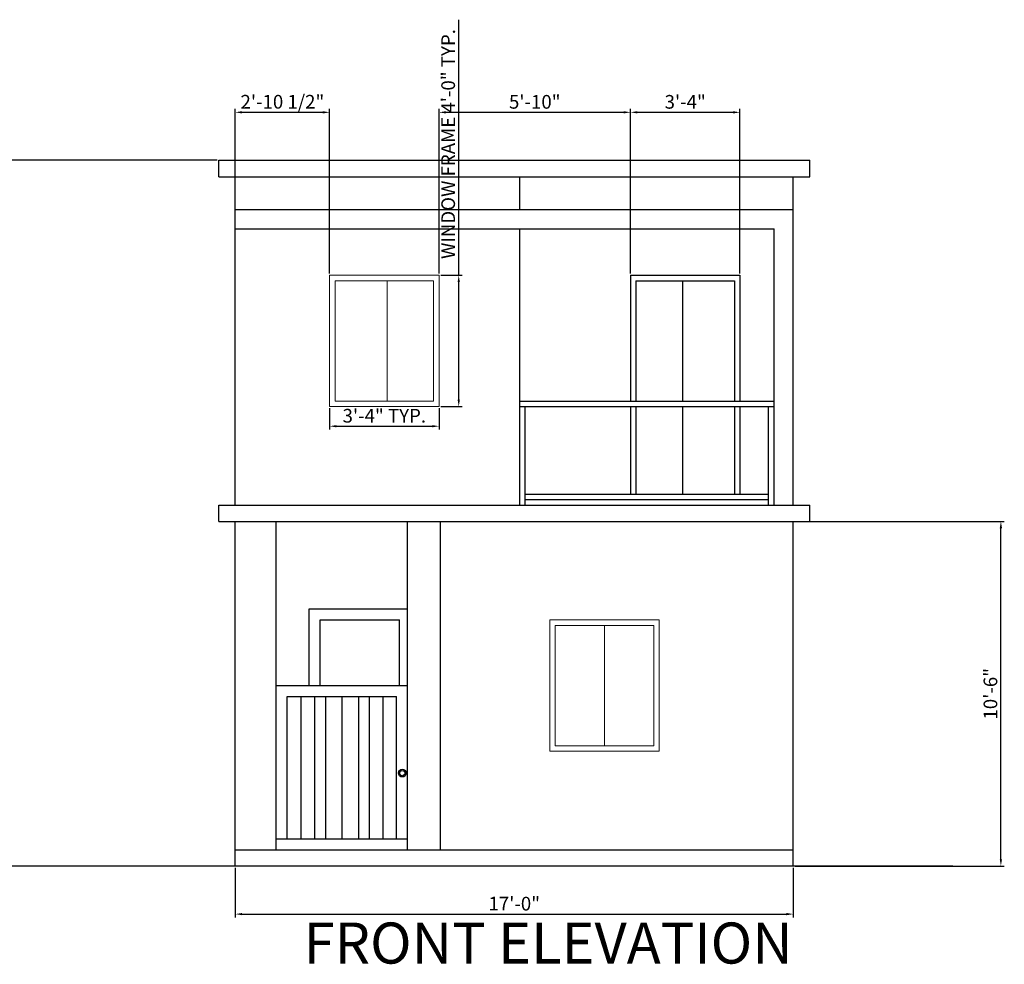
# Model space of a CAD drawing. Units: inches. Extents: x 1662 to 23131, y 1265 to 19127.
# Tile 17 of 26: x 20050 to 20410, y 8426 to 8771. Entities that reach past the tile are written whole.
import ezdxf

# ---------------------------------------------------------------- set-up
doc = ezdxf.new("R2010")
doc.units = ezdxf.units.IN
for name, color, linetype, lineweight in [('A-ANNO-DIMS', 4, 'Continuous', 18), ('A-ANNO-TITL', 7, 'Continuous', 35), ('A-ELEV', 7, 'Continuous', 25), ('A-ELEV-GLAZ', 4, 'Continuous', 18)]:
    doc.layers.add(name, color=color, linetype=linetype, lineweight=lineweight)
doc.styles.get("Standard").update_dxf_attribs({"font": 'arial.ttf'})
doc.dimstyles.new('ISO-25', dxfattribs={"dimtxt": 5, "dimasz": 2.5, "dimexe": 1.25, "dimexo": 0.625, "dimtad": 1, "dimlunit": 3, "dimtxsty": 'Standard', "dimcen": 2.5, "dimadec": 0, "dimazin": 0, "dimtfac": 1, "dimtmove": 0, "dimatfit": 3, "dimfxl": 1, "dimarcsym": 0})

# ---------------------------------------------------------------- blocks, each defined once
blk = doc.blocks.new('GLAZ-FRAME-ELEV-40X48')
for p, q in [((0, 48), (0, 0)), ((40, 48), (0, 48)), ((40, 48), (40, 0)), ((2, 46), (2, 2)), ((38, 46), (2, 46)), ((38, 46), (38, 2)), ((38, 2), (2, 2)), ((40, 0), (0, 0))]:
    blk.add_line(p, q)
blk = doc.blocks.new('*D195')
at = {"layer": 'A-ANNO-DIMS', "color": 0, "lineweight": -2, "transparency": 16777216}
for p, q in [((20210.7, 8677.94), (20210.7, 8771.35)), ((20204.13, 8677.94), (20211.95, 8677.94)), ((20210.7, 8632.44), (20210.7, 8675.44)), ((20204.13, 8629.94), (20211.95, 8629.94))]:
    blk.add_line(p, q, dxfattribs=at)
at = {"layer": 'A-ANNO-DIMS', "color": 0, "transparency": 16777216}
for points in [[(20210.29, 8675.44), (20211.12, 8675.44), (20210.7, 8677.94)], [(20210.29, 8632.44), (20211.12, 8632.44), (20210.7, 8629.94)]]:
    blk.add_solid(points, dxfattribs=at)
at = {"layer": 'Defpoints', "color": 0, "transparency": 16777216}
for p in [(20203.5, 8677.94), (20210.7, 8677.94), (20203.5, 8629.94)]:
    blk.add_point(p, dxfattribs=at)
at = {"layer": 'A-ANNO-DIMS', "color": 0, "transparency": 16777216, "insert": (20207.49, 8725.89), "char_height": 5, "attachment_point": 5, "rotation": 90}
blk.add_mtext('WINDOW FRAME 4\'-0" TYP.', dxfattribs=at)
blk = doc.blocks.new('*D196')
at = {"layer": 'A-ANNO-DIMS', "color": 0, "lineweight": -2, "transparency": 16777216}
for p, q in [((20163.5, 8629.31), (20163.5, 8621.49)), ((20203.5, 8629.31), (20203.5, 8621.49)), ((20166, 8622.74), (20201, 8622.74))]:
    blk.add_line(p, q, dxfattribs=at)
at = {"layer": 'A-ANNO-DIMS', "color": 0, "transparency": 16777216}
for points in [[(20166, 8623.16), (20166, 8622.32), (20163.5, 8622.74)], [(20201, 8623.16), (20201, 8622.32), (20203.5, 8622.74)]]:
    blk.add_solid(points, dxfattribs=at)
at = {"layer": 'Defpoints', "color": 0, "transparency": 16777216}
for p in [(20163.5, 8629.94), (20203.5, 8629.94), (20203.5, 8622.74)]:
    blk.add_point(p, dxfattribs=at)
at = {"layer": 'A-ANNO-DIMS', "color": 0, "transparency": 16777216, "insert": (20183.5, 8625.92), "char_height": 5, "attachment_point": 5}
blk.add_mtext('3\'-4" TYP.', dxfattribs=at)
blk = doc.blocks.new('*D245')
at = {"layer": 'A-ANNO-DIMS', "color": 0, "lineweight": -2, "transparency": 16777216}
for p, q in [((20129, 8461.31), (20129, 8443.14)), ((20333, 8461.31), (20333, 8443.14)), ((20131.5, 8444.39), (20330.5, 8444.39))]:
    blk.add_line(p, q, dxfattribs=at)
at = {"layer": 'A-ANNO-DIMS', "color": 0, "transparency": 16777216}
for points in [[(20131.5, 8444.81), (20131.5, 8443.97), (20129, 8444.39)], [(20330.5, 8444.81), (20330.5, 8443.97), (20333, 8444.39)]]:
    blk.add_solid(points, dxfattribs=at)
at = {"layer": 'Defpoints', "color": 0, "transparency": 16777216}
for p in [(20129, 8461.94), (20333, 8461.94), (20333, 8444.39)]:
    blk.add_point(p, dxfattribs=at)
at = {"layer": 'A-ANNO-DIMS', "color": 0, "transparency": 16777216, "insert": (20231, 8447.57), "char_height": 5, "attachment_point": 5}
blk.add_mtext('17\'-0"', dxfattribs=at)
blk = doc.blocks.new('*D246')
at = {"layer": 'A-ANNO-DIMS', "color": 0, "lineweight": -2, "transparency": 16777216}
for p, q in [((20122.38, 8719.94), (20031.81, 8719.94)), ((20033.06, 8464.44), (20033.06, 8717.44)), ((20128.38, 8461.94), (20031.81, 8461.94))]:
    blk.add_line(p, q, dxfattribs=at)
at = {"layer": 'A-ANNO-DIMS', "color": 0, "transparency": 16777216}
for points in [[(20032.64, 8717.44), (20033.48, 8717.44), (20033.06, 8719.94)], [(20032.64, 8464.44), (20033.48, 8464.44), (20033.06, 8461.94)]]:
    blk.add_solid(points, dxfattribs=at)
at = {"layer": 'Defpoints', "color": 0, "transparency": 16777216}
for p in [(20033.06, 8719.94), (20123, 8719.94), (20129, 8461.94)]:
    blk.add_point(p, dxfattribs=at)
at = {"layer": 'A-ANNO-DIMS', "color": 0, "transparency": 16777216, "insert": (20029.88, 8590.94), "char_height": 5, "attachment_point": 5, "rotation": 90}
blk.add_mtext('21\'-6"', dxfattribs=at)
blk = doc.blocks.new('*D247')
at = {"layer": 'A-ANNO-DIMS', "color": 0, "lineweight": -2, "transparency": 16777216}
for p, q in [((20333.63, 8587.94), (20410.14, 8587.94)), ((20408.89, 8464.44), (20408.89, 8585.44)), ((20333.63, 8461.94), (20410.14, 8461.94))]:
    blk.add_line(p, q, dxfattribs=at)
at = {"layer": 'A-ANNO-DIMS', "color": 0, "transparency": 16777216}
for points in [[(20408.48, 8585.44), (20409.31, 8585.44), (20408.89, 8587.94)], [(20408.48, 8464.44), (20409.31, 8464.44), (20408.89, 8461.94)]]:
    blk.add_solid(points, dxfattribs=at)
at = {"layer": 'Defpoints', "color": 0, "transparency": 16777216}
for p in [(20333, 8587.94), (20408.89, 8587.94), (20333, 8461.94)]:
    blk.add_point(p, dxfattribs=at)
at = {"layer": 'A-ANNO-DIMS', "color": 0, "transparency": 16777216, "insert": (20405.72, 8524.94), "char_height": 5, "attachment_point": 5, "rotation": 90}
blk.add_mtext('10\'-6"', dxfattribs=at)
blk = doc.blocks.new('*D248')
at = {"layer": 'A-ANNO-DIMS', "color": 0, "lineweight": -2, "transparency": 16777216}
for p, q in [((20203.5, 8678.56), (20203.5, 8738.74)), ((20206, 8737.49), (20271, 8737.49)), ((20273.5, 8678.56), (20273.5, 8738.74))]:
    blk.add_line(p, q, dxfattribs=at)
at = {"layer": 'A-ANNO-DIMS', "color": 0, "transparency": 16777216}
for points in [[(20206, 8737.91), (20206, 8737.07), (20203.5, 8737.49)], [(20271, 8737.91), (20271, 8737.07), (20273.5, 8737.49)]]:
    blk.add_solid(points, dxfattribs=at)
at = {"layer": 'Defpoints', "color": 0, "transparency": 16777216}
for p in [(20273.5, 8737.49), (20203.5, 8677.94), (20273.5, 8677.94)]:
    blk.add_point(p, dxfattribs=at)
at = {"layer": 'A-ANNO-DIMS', "color": 0, "transparency": 16777216, "insert": (20238.5, 8740.67), "char_height": 5, "attachment_point": 5}
blk.add_mtext('5\'-10"', dxfattribs=at)
blk = doc.blocks.new('*D249')
at = {"layer": 'A-ANNO-DIMS', "color": 0, "lineweight": -2, "transparency": 16777216}
for p, q in [((20129, 8695.56), (20129, 8738.74)), ((20131.5, 8737.49), (20161, 8737.49)), ((20163.5, 8678.56), (20163.5, 8738.74))]:
    blk.add_line(p, q, dxfattribs=at)
at = {"layer": 'A-ANNO-DIMS', "color": 0, "transparency": 16777216}
for points in [[(20131.5, 8737.91), (20131.5, 8737.07), (20129, 8737.49)], [(20161, 8737.91), (20161, 8737.07), (20163.5, 8737.49)]]:
    blk.add_solid(points, dxfattribs=at)
at = {"layer": 'Defpoints', "color": 0, "transparency": 16777216}
for p in [(20163.5, 8737.49), (20129, 8694.94), (20163.5, 8677.94)]:
    blk.add_point(p, dxfattribs=at)
at = {"layer": 'A-ANNO-DIMS', "color": 0, "transparency": 16777216, "insert": (20146.25, 8740.7), "char_height": 5, "attachment_point": 5}
blk.add_mtext('2\'-10 1/2"', dxfattribs=at)
blk = doc.blocks.new('*D250')
at = {"layer": 'A-ANNO-DIMS', "color": 0, "lineweight": -2, "transparency": 16777216}
for p, q in [((20273.5, 8678.56), (20273.5, 8738.74)), ((20276, 8737.49), (20311, 8737.49)), ((20313.5, 8678.56), (20313.5, 8738.74))]:
    blk.add_line(p, q, dxfattribs=at)
at = {"layer": 'A-ANNO-DIMS', "color": 0, "transparency": 16777216}
for points in [[(20276, 8737.91), (20276, 8737.07), (20273.5, 8737.49)], [(20311, 8737.91), (20311, 8737.07), (20313.5, 8737.49)]]:
    blk.add_solid(points, dxfattribs=at)
at = {"layer": 'Defpoints', "color": 0, "transparency": 16777216}
for p in [(20313.5, 8737.49), (20273.5, 8677.94), (20313.5, 8677.94)]:
    blk.add_point(p, dxfattribs=at)
at = {"layer": 'A-ANNO-DIMS', "color": 0, "transparency": 16777216, "insert": (20293.5, 8740.67), "char_height": 5, "attachment_point": 5}
blk.add_mtext('3\'-4"', dxfattribs=at)

msp = doc.modelspace()

# ---------------------------------------------------------------- linework, layer by layer
at = {"layer": 'A-ELEV'}
for p, q in [((20123.002, 8719.939), (20339.002, 8719.939)), ((20123.002, 8713.939), (20123.002, 8719.939)), ((20339.002, 8713.939), (20339.002, 8719.939)), ((20123.002, 8713.939), (20339.002, 8713.939)), ((20129.002, 8593.939), (20129.002, 8713.939)), ((20233.002, 8701.939), (20233.002, 8713.939)), ((20333.002, 8593.939), (20333.002, 8713.939)), ((20129.002, 8701.939), (20333.002, 8701.939)), ((20129.002, 8694.939), (20326.002, 8694.939)), ((20233.002, 8593.939), (20233.002, 8694.939)), ((20326.002, 8593.939), (20326.002, 8694.939)), ((20273.502, 8677.939), (20273.502, 8631.939)), ((20273.502, 8677.939), (20313.502, 8677.939)), ((20275.502, 8675.939), (20275.502, 8631.939)), ((20275.502, 8675.939), (20311.502, 8675.939)), ((20292.502, 8675.939), (20292.502, 8631.939)), ((20311.502, 8675.939), (20311.502, 8631.939)), ((20313.502, 8677.939), (20313.502, 8631.939)), ((20233.002, 8631.939), (20326.002, 8631.939)), ((20233.002, 8629.939), (20326.002, 8629.939)), ((20235.002, 8593.939), (20235.002, 8629.939)), ((20273.502, 8629.939), (20273.502, 8597.939)), ((20275.502, 8629.939), (20275.502, 8597.939)), ((20292.502, 8629.939), (20292.502, 8597.939)), ((20311.502, 8629.939), (20311.502, 8597.939)), ((20313.502, 8629.939), (20313.502, 8597.939)), ((20313.502, 8629.939), (20313.502, 8597.939)), ((20324.002, 8593.939), (20324.002, 8629.939)), ((20235.002, 8597.939), (20324.002, 8597.939)), ((20235.002, 8595.939), (20324.002, 8595.939)), ((20123.002, 8593.939), (20339.002, 8593.939)), ((20123.002, 8587.939), (20123.002, 8593.939)), ((20339.002, 8587.939), (20339.002, 8593.939)), ((20123.002, 8587.939), (20339.002, 8587.939)), ((20129.002, 8461.939), (20129.002, 8587.939)), ((20144.002, 8467.939), (20144.002, 8587.939)), ((20192.002, 8467.939), (20192.002, 8587.939)), ((20204.002, 8467.939), (20204.002, 8587.939)), ((20333.002, 8461.939), (20333.002, 8587.939)), ((20156.002, 8527.939), (20156.002, 8555.939)), ((20156.002, 8555.939), (20192.002, 8555.939)), ((20160.002, 8551.939), (20189.002, 8551.939)), ((20160.002, 8527.939), (20160.002, 8551.939)), ((20189.002, 8527.939), (20189.002, 8551.939)), ((20144.002, 8527.939), (20192.002, 8527.939)), ((20148.002, 8471.939), (20148.002, 8523.939)), ((20148.002, 8523.939), (20188.002, 8523.939)), ((20153.002, 8523.939), (20153.002, 8471.939)), ((20158.002, 8523.939), (20158.002, 8471.939)), ((20162.002, 8523.939), (20162.002, 8471.939)), ((20168.002, 8523.939), (20168.002, 8471.939)), ((20174.002, 8523.939), (20174.002, 8471.939)), ((20178.002, 8523.939), (20178.002, 8471.939)), ((20183.002, 8523.939), (20183.002, 8471.939)), ((20188.002, 8471.939), (20188.002, 8523.939)), ((20144.002, 8471.939), (20192.002, 8471.939)), ((20129.002, 8467.939), (20333.002, 8467.939)), ((20391.344, 8461.939), (20050.611, 8461.939)), ((20391.344, 8461.939), (20391.344, 8461.939))]:
    msp.add_line(p, q, dxfattribs=at)
for radius in [1.424, 0.953]:
    msp.add_circle((20190.068, 8495.939), radius, dxfattribs=at)
at = {"layer": 'A-ELEV-GLAZ'}
for p, q in [((20184.502, 8675.939), (20184.502, 8631.939)), ((20264.002, 8549.939), (20264.002, 8505.939))]:
    msp.add_line(p, q, dxfattribs=at)

# ---------------------------------------------------------------- block references
msp.add_blockref('GLAZ-FRAME-ELEV-40X48', (20163.502, 8629.939), dxfattribs=at)
at = {"layer": 'A-ELEV-GLAZ', "rotation": 180}
msp.add_blockref('GLAZ-FRAME-ELEV-40X48', (20284.001, 8551.939), dxfattribs=at)

# ---------------------------------------------------------------- texts
at = {"layer": 'A-ANNO-TITL', "insert": (20154.009, 8441.307), "char_height": 15, "attachment_point": 1}
msp.add_mtext_dynamic_manual_height_columns('FRONT ELEVATION', width=1142.59551, gutter_width=12.5, heights=[0], dxfattribs=at)

# ---------------------------------------------------------------- dimensions: what is measured, and where the dimension line sits
at = {"layer": 'A-ANNO-DIMS'}
dim = msp.add_linear_dim(base=(20210.702, 8677.939), p1=(20203.502, 8629.939), p2=(20203.502, 8677.939), angle=90, text='WINDOW FRAME <> TYP.', dimstyle='ISO-25', override={"dimdec": 1, "dimlfac": 1, "dimrnd": 0, "dimzin": 1, "dimdsep": 46, "dimlunit": 4, "dimfrac": 2}, dxfattribs=at)
dim.commit()
dim.dimension.update_dxf_attribs({"geometry": '*D195', "text_midpoint": (20207.49, 8725.893)})
for base, p1, p2, picture, middle in [((20163.502, 8737.489), (20129.002, 8694.939), (20163.502, 8677.939), '*D249', (20146.252, 8740.699)), ((20273.502, 8737.489), (20203.502, 8677.939), (20273.502, 8677.939), '*D248', (20238.502, 8740.667)), ((20313.502, 8737.489), (20273.502, 8677.939), (20313.502, 8677.939), '*D250', (20293.502, 8740.668)), ((20333.002, 8444.389), (20129.002, 8461.939), (20333.002, 8461.939), '*D245', (20231.002, 8447.567))]:
    dim = msp.add_linear_dim(base=base, p1=p1, p2=p2, dimstyle='ISO-25', override={"dimdec": 1, "dimlfac": 1, "dimrnd": 0, "dimzin": 1, "dimdsep": 46, "dimlunit": 4, "dimfrac": 2}, dxfattribs=at)
    dim.commit()
    dim.dimension.update_dxf_attribs({"geometry": picture, "text_midpoint": middle})
for base, p1, p2, picture, middle in [((20033.061, 8719.939), (20129.002, 8461.939), (20123.002, 8719.939), '*D246', (20029.883, 8590.939)), ((20408.894, 8587.939), (20333.002, 8461.939), (20333.002, 8587.939), '*D247', (20405.716, 8524.939))]:
    dim = msp.add_linear_dim(base=base, p1=p1, p2=p2, angle=90, dimstyle='ISO-25', override={"dimdec": 1, "dimlfac": 1, "dimrnd": 0, "dimzin": 1, "dimdsep": 46, "dimlunit": 4, "dimfrac": 2}, dxfattribs=at)
    dim.commit()
    dim.dimension.update_dxf_attribs({"geometry": picture, "text_midpoint": middle})
dim = msp.add_linear_dim(base=(20203.502, 8622.739), p1=(20163.502, 8629.939), p2=(20203.502, 8629.939), text='<> TYP.', dimstyle='ISO-25', override={"dimdec": 1, "dimlfac": 1, "dimrnd": 0, "dimzin": 1, "dimdsep": 46, "dimlunit": 4, "dimfrac": 2}, dxfattribs=at)
dim.commit()
dim.dimension.update_dxf_attribs({"geometry": '*D196', "text_midpoint": (20183.502, 8625.918)})

doc.saveas('drawing.dxf')
